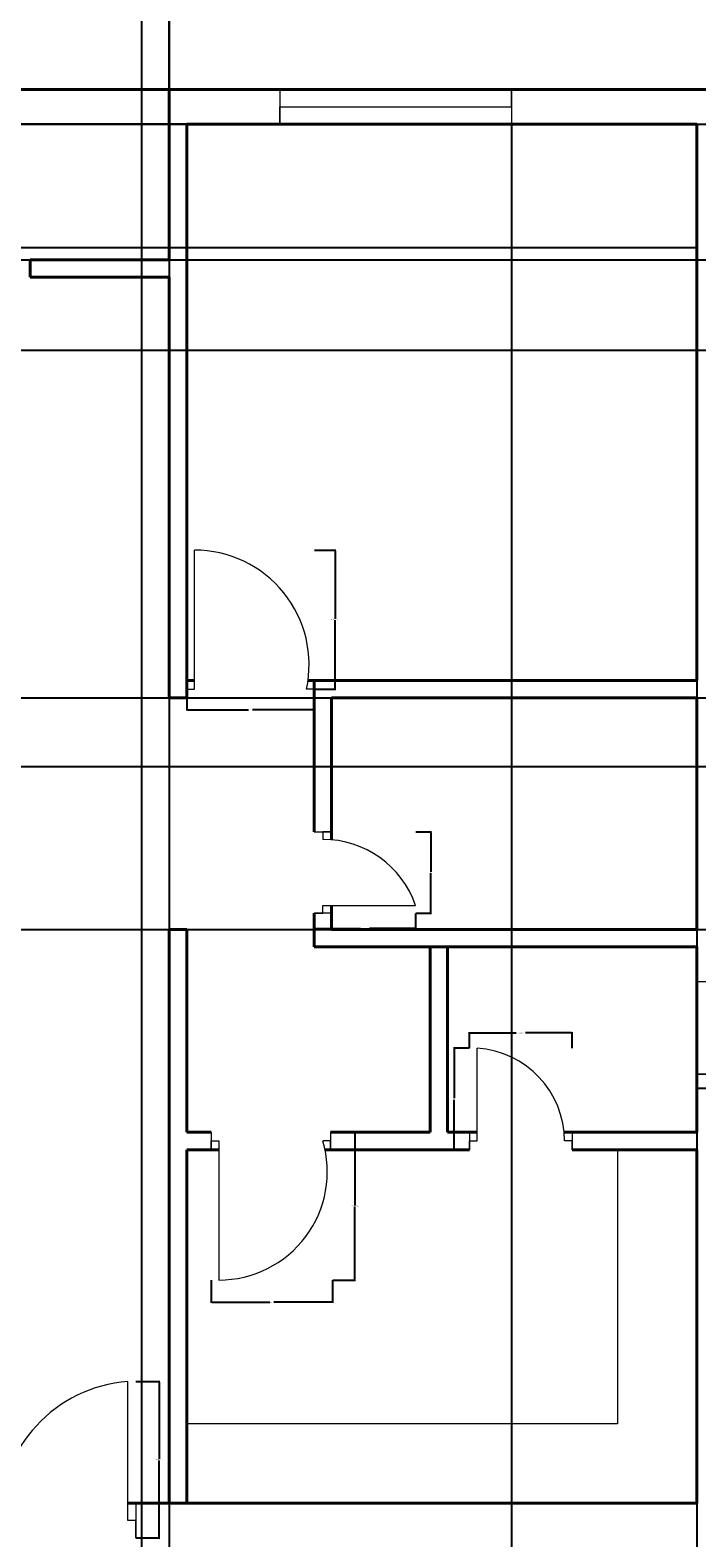
# Model space of a CAD drawing. Units: inches. Extents: x 1355 to 2746, y 1171 to 2751.
# Tile 17 of 24: x 2325 to 2497, y 1764 to 2155. Entities that reach past the tile are written whole.
import ezdxf

# ---------------------------------------------------------------- set-up
doc = ezdxf.new("R2010")
doc.units = ezdxf.units.IN
for name, color, linetype, lineweight in [('A-ANNO-DIMS', 2, 'Continuous', 18), ('A-DOOR', 3, 'Continuous', 20), ('A-FLOR-CASE', 30, 'Continuous', 20), ('A-GLAZ', 4, 'Continuous', 18), ('A-WALL', 7, 'Continuous', 40)]:
    doc.layers.add(name, color=color, linetype=linetype, lineweight=lineweight)
doc.styles.get("Standard").update_dxf_attribs({"font": 'arial.ttf'})
doc.dimstyles.get("Standard").update_dxf_attribs({"dimtxt": 0.18, "dimasz": 0.18, "dimexe": 0.18, "dimexo": 0.0625, "dimgap": 0.09, "dimtad": 0, "dimtih": 1, "dimtoh": 1, "dimdec": 4, "dimzin": 0, "dimdsep": 46, "dimtxsty": 'Standard', "dimcen": 0.09, "dimadec": 0, "dimazin": 0, "dimtfac": 1, "dimtdec": 4, "dimtofl": 0, "dimtmove": 0, "dimatfit": 3, "dimfxl": 1, "dimtolj": 1, "dimtzin": 0, "dimarcsym": 0})

# ---------------------------------------------------------------- blocks, each defined once
blk = doc.blocks.new('WINDOW-PLAN-24-2')
for p, q in [((0, 24), (9, 24)), ((9, 24), (4.5, 24)), ((4.5, 24), (4.5, 0)), ((4.5, 0), (0, 0)), ((0, 0), (0, 0)), ((0, 0), (9, 0))]:
    blk.add_line(p, q)
blk = doc.blocks.new('WINDOW-PLAN-60')
for p, q in [((0, 60), (9, 60)), ((9, 60), (4.5, 60)), ((4.5, 60), (4.5, 0)), ((4.5, 0), (0, 0)), ((0, 0), (9, 0))]:
    blk.add_line(p, q)
blk = doc.blocks.new('DOOR-ENTRY-N')
for p, q in [((35.29, 4.5), (35.29, 40.5)), ((0, 9), (0, 0)), ((37.29, 9), (37.29, 0)), ((0, 0), (0, 4.5)), ((0, 4.5), (2, 4.5)), ((37.29, 4.5), (35.29, 4.5)), ((37.29, 0), (37.29, 4.5))]:
    blk.add_line(p, q)
blk.add_arc((38.11, 4.5), 36.11, 94.4716, 180)
blk = doc.blocks.new('DOOR-UTILITY-N')
for p, q in [((2, 2.25), (2, 26.25)), ((0, 4.5), (0, 0)), ((26.56, 4.5), (26.56, 0)), ((0, 0), (0, 2.25)), ((0, 2.25), (2, 2.25)), ((26.56, 2.25), (24.56, 2.25)), ((26.56, 0), (26.56, 2.25))]:
    blk.add_line(p, q)
blk.add_arc((0.51, 2.25), 24.05, 0, 86.4557)
blk = doc.blocks.new('DOOR-KITCHEN-N')
for p, q in [((0, 38.25), (0, 33.75)), ((0, 33.75), (0, 36)), ((0, 36), (2, 36)), ((2, 36), (2, 0)), ((30.9, 36), (28.9, 36)), ((30.9, 38.25), (30.9, 33.75)), ((30.9, 33.75), (30.9, 36))]:
    blk.add_line(p, q)
blk.add_arc((2, 28.05), 28.05, 270, 16.4594)
blk = doc.blocks.new('DOOR-BED-NE')
for p, q in [((2, 0), (2, 36)), ((33, 0.01), (31, 0.01)), ((0, 0), (2, 0))]:
    blk.add_line(p, q)
blk.add_arc((2, 6.32), 29.68, 347.7257, 90)
blk = doc.blocks.new('DOOR-WC-NE')
for p, q in [((0, 21.08), (4.5, 21.08)), ((4.5, 21.08), (2.25, 21.08)), ((2.25, 21.08), (2.25, 19.08)), ((4.5, 0), (0, 0)), ((0, 0), (2.25, 0)), ((2.25, 0), (2.25, 2)), ((2.25, 2), (26.25, 2))]:
    blk.add_line(p, q)
blk.add_arc((2.25, -6.32), 25.4, 19.1149, 90)
blk = doc.blocks.new('*D50')
at = {"layer": 'A-ANNO-DIMS', "color": 0, "lineweight": -2, "transparency": 16777216}
for p, q in [((2497.39, 1884.27), (2497.39, 1880.55)), ((2506.39, 1884.27), (2506.39, 1880.55)), ((2497.57, 1880.73), (2501.43, 1880.73)), ((2506.21, 1880.73), (2502.35, 1880.73))]:
    blk.add_line(p, q, dxfattribs=at)
at = {"layer": 'A-ANNO-DIMS', "color": 0, "transparency": 16777216}
for points in [[(2497.57, 1880.76), (2497.57, 1880.7), (2497.39, 1880.73)], [(2506.21, 1880.76), (2506.21, 1880.7), (2506.39, 1880.73)]]:
    blk.add_solid(points, dxfattribs=at)
at = {"layer": 'Defpoints', "color": 0, "transparency": 16777216}
for p in [(2497.39, 1884.33), (2506.39, 1884.33), (2506.39, 1880.73)]:
    blk.add_point(p, dxfattribs=at)
at = {"layer": 'A-ANNO-DIMS', "color": 0, "transparency": 16777216, "insert": (2501.89, 1880.73), "char_height": 0.18, "attachment_point": 5}
blk.add_mtext('\\A1;9 TYP.', dxfattribs=at)
blk = doc.blocks.new('*D55')
at = {"layer": 'A-ANNO-DIMS', "color": 0, "lineweight": -2, "transparency": 16777216}
for p, q in [((2352.26, 1804.8), (2358.45, 1804.8)), ((2358.27, 1804.62), (2358.27, 1784.73)), ((2358.27, 1764.48), (2358.27, 1784.37)), ((2352.26, 1764.3), (2358.45, 1764.3))]:
    blk.add_line(p, q, dxfattribs=at)
at = {"layer": 'A-ANNO-DIMS', "color": 0, "transparency": 16777216}
for points in [[(2358.24, 1804.62), (2358.3, 1804.62), (2358.27, 1804.8)], [(2358.24, 1764.48), (2358.3, 1764.48), (2358.27, 1764.3)]]:
    blk.add_solid(points, dxfattribs=at)
at = {"layer": 'Defpoints', "color": 0, "transparency": 16777216}
for p in [(2352.2, 1804.8), (2358.27, 1804.8), (2352.2, 1764.3)]:
    blk.add_point(p, dxfattribs=at)
at = {"layer": 'A-ANNO-DIMS', "color": 0, "transparency": 16777216, "insert": (2358.27, 1784.55), "char_height": 0.18, "attachment_point": 5}
blk.add_mtext('\\A1;ENTRY DOOR 41 TYP.', dxfattribs=at)
blk = doc.blocks.new('*D57')
at = {"layer": 'A-ANNO-DIMS', "color": 0, "lineweight": -2, "transparency": 16777216}
for p, q in [((2438.58, 1891.11), (2438.58, 1895.22)), ((2438.76, 1895.04), (2450.62, 1895.04)), ((2464.96, 1895.04), (2453.1, 1895.04)), ((2465.14, 1891.11), (2465.14, 1895.22))]:
    blk.add_line(p, q, dxfattribs=at)
at = {"layer": 'A-ANNO-DIMS', "color": 0, "transparency": 16777216}
for points in [[(2438.76, 1895.07), (2438.76, 1895.01), (2438.58, 1895.04)], [(2464.96, 1895.07), (2464.96, 1895.01), (2465.14, 1895.04)]]:
    blk.add_solid(points, dxfattribs=at)
at = {"layer": 'Defpoints', "color": 0, "transparency": 16777216}
for p in [(2465.14, 1895.04), (2438.58, 1891.05), (2465.14, 1891.05)]:
    blk.add_point(p, dxfattribs=at)
at = {"layer": 'A-ANNO-DIMS', "color": 0, "transparency": 16777216, "insert": (2451.86, 1895.04), "char_height": 0.18, "attachment_point": 5}
blk.add_mtext('\\A1;UTIL DOOR 27 TYP.', dxfattribs=at)
blk = doc.blocks.new('*D58')
at = {"layer": 'A-ANNO-DIMS', "color": 0, "lineweight": -2, "transparency": 16777216}
for p, q in [((2438.52, 1891.05), (2434.42, 1891.05)), ((2434.6, 1890.87), (2434.6, 1878.11)), ((2434.6, 1864.98), (2434.6, 1877.74)), ((2438.52, 1864.8), (2434.42, 1864.8))]:
    blk.add_line(p, q, dxfattribs=at)
at = {"layer": 'A-ANNO-DIMS', "color": 0, "transparency": 16777216}
for points in [[(2434.57, 1890.87), (2434.63, 1890.87), (2434.6, 1891.05)], [(2434.57, 1864.98), (2434.63, 1864.98), (2434.6, 1864.8)]]:
    blk.add_solid(points, dxfattribs=at)
at = {"layer": 'Defpoints', "color": 0, "transparency": 16777216}
for p in [(2434.6, 1891.05), (2438.58, 1891.05), (2438.58, 1864.8)]:
    blk.add_point(p, dxfattribs=at)
at = {"layer": 'A-ANNO-DIMS', "color": 0, "transparency": 16777216, "insert": (2434.6, 1877.93), "char_height": 0.18, "attachment_point": 5}
blk.add_mtext('\\A1;26 TYP.', dxfattribs=at)
blk = doc.blocks.new('*D59')
at = {"layer": 'A-ANNO-DIMS', "color": 0, "lineweight": -2, "transparency": 16777216}
for p, q in [((2403.21, 1869.3), (2409.06, 1869.3)), ((2408.88, 1869.12), (2408.88, 1850.36)), ((2408.88, 1831.23), (2408.88, 1849.99)), ((2403.21, 1831.05), (2409.06, 1831.05))]:
    blk.add_line(p, q, dxfattribs=at)
at = {"layer": 'A-ANNO-DIMS', "color": 0, "transparency": 16777216}
for points in [[(2408.85, 1869.12), (2408.91, 1869.12), (2408.88, 1869.3)], [(2408.85, 1831.23), (2408.91, 1831.23), (2408.88, 1831.05)]]:
    blk.add_solid(points, dxfattribs=at)
at = {"layer": 'Defpoints', "color": 0, "transparency": 16777216}
for p in [(2403.14, 1869.3), (2408.88, 1869.3), (2403.14, 1831.05)]:
    blk.add_point(p, dxfattribs=at)
at = {"layer": 'A-ANNO-DIMS', "color": 0, "transparency": 16777216, "insert": (2408.88, 1850.18), "char_height": 0.18, "attachment_point": 5}
blk.add_mtext('\\A1;KIT DOOR 38 TYP.', dxfattribs=at)
blk = doc.blocks.new('*D60')
at = {"layer": 'A-ANNO-DIMS', "color": 0, "lineweight": -2, "transparency": 16777216}
for p, q in [((2371.73, 1830.99), (2371.73, 1825.13)), ((2403.14, 1830.99), (2403.14, 1825.13)), ((2371.91, 1825.31), (2386.91, 1825.31)), ((2402.96, 1825.31), (2387.97, 1825.31))]:
    blk.add_line(p, q, dxfattribs=at)
at = {"layer": 'A-ANNO-DIMS', "color": 0, "transparency": 16777216}
for points in [[(2371.91, 1825.34), (2371.91, 1825.28), (2371.73, 1825.31)], [(2402.96, 1825.34), (2402.96, 1825.28), (2403.14, 1825.31)]]:
    blk.add_solid(points, dxfattribs=at)
at = {"layer": 'Defpoints', "color": 0, "transparency": 16777216}
for p in [(2371.73, 1831.05), (2403.14, 1831.05), (2403.14, 1825.31)]:
    blk.add_point(p, dxfattribs=at)
at = {"layer": 'A-ANNO-DIMS', "color": 0, "transparency": 16777216, "insert": (2387.44, 1825.31), "char_height": 0.18, "attachment_point": 5}
blk.add_mtext('\\A1;31 TYP.', dxfattribs=at)
blk = doc.blocks.new('*D77')
at = {"layer": 'A-ANNO-DIMS', "color": 0, "lineweight": -2, "transparency": 16777216}
for p, q in [((2398.45, 2020.05), (2403.97, 2020.05)), ((2403.79, 2019.87), (2403.79, 2002.24)), ((2403.79, 1984.23), (2403.79, 2001.87)), ((2398.45, 1984.05), (2403.97, 1984.05))]:
    blk.add_line(p, q, dxfattribs=at)
at = {"layer": 'A-ANNO-DIMS', "color": 0, "transparency": 16777216}
for points in [[(2403.76, 2019.87), (2403.82, 2019.87), (2403.79, 2020.05)], [(2403.76, 1984.23), (2403.82, 1984.23), (2403.79, 1984.05)]]:
    blk.add_solid(points, dxfattribs=at)
at = {"layer": 'Defpoints', "color": 0, "transparency": 16777216}
for p in [(2398.39, 2020.05), (2403.79, 2020.05), (2398.39, 1984.05)]:
    blk.add_point(p, dxfattribs=at)
at = {"layer": 'A-ANNO-DIMS', "color": 0, "transparency": 16777216, "insert": (2403.79, 2002.05), "char_height": 0.18, "attachment_point": 5}
blk.add_mtext('\\A1;BED DOOR 36 TYP.', dxfattribs=at)
blk = doc.blocks.new('*D78')
at = {"layer": 'A-ANNO-DIMS', "color": 0, "lineweight": -2, "transparency": 16777216}
for p, q in [((2365.39, 1983.99), (2365.39, 1978.47)), ((2398.39, 1983.99), (2398.39, 1978.47)), ((2365.57, 1978.65), (2381.36, 1978.65)), ((2398.21, 1978.65), (2382.42, 1978.65))]:
    blk.add_line(p, q, dxfattribs=at)
at = {"layer": 'A-ANNO-DIMS', "color": 0, "transparency": 16777216}
for points in [[(2365.57, 1978.68), (2365.57, 1978.62), (2365.39, 1978.65)], [(2398.21, 1978.68), (2398.21, 1978.62), (2398.39, 1978.65)]]:
    blk.add_solid(points, dxfattribs=at)
at = {"layer": 'Defpoints', "color": 0, "transparency": 16777216}
for p in [(2365.39, 1984.05), (2398.39, 1984.05), (2398.39, 1978.65)]:
    blk.add_point(p, dxfattribs=at)
at = {"layer": 'A-ANNO-DIMS', "color": 0, "transparency": 16777216, "insert": (2381.89, 1978.65), "char_height": 0.18, "attachment_point": 5}
blk.add_mtext('\\A1;33 TYP.', dxfattribs=at)
blk = doc.blocks.new('*D79')
at = {"layer": 'A-ANNO-DIMS', "color": 0, "lineweight": -2, "transparency": 16777216}
for p, q in [((2398.39, 1925.99), (2398.39, 1921.93)), ((2424.64, 1925.99), (2424.64, 1921.93)), ((2398.57, 1922.11), (2410.33, 1922.11)), ((2424.46, 1922.11), (2412.7, 1922.11))]:
    blk.add_line(p, q, dxfattribs=at)
at = {"layer": 'A-ANNO-DIMS', "color": 0, "transparency": 16777216}
for points in [[(2398.57, 1922.14), (2398.57, 1922.08), (2398.39, 1922.11)], [(2424.46, 1922.14), (2424.46, 1922.08), (2424.64, 1922.11)]]:
    blk.add_solid(points, dxfattribs=at)
at = {"layer": 'Defpoints', "color": 0, "transparency": 16777216}
for p in [(2398.39, 1926.05), (2424.64, 1926.05), (2424.64, 1922.11)]:
    blk.add_point(p, dxfattribs=at)
at = {"layer": 'A-ANNO-DIMS', "color": 0, "transparency": 16777216, "insert": (2411.52, 1922.11), "char_height": 0.18, "attachment_point": 5}
blk.add_mtext('\\A1;WC DOOR 26 TYP.', dxfattribs=at)
blk = doc.blocks.new('*D80')
at = {"layer": 'A-ANNO-DIMS', "color": 0, "lineweight": -2, "transparency": 16777216}
for p, q in [((2424.7, 1947.13), (2428.76, 1947.13)), ((2428.58, 1946.95), (2428.58, 1936.77)), ((2428.58, 1926.23), (2428.58, 1936.41)), ((2424.7, 1926.05), (2428.76, 1926.05))]:
    blk.add_line(p, q, dxfattribs=at)
at = {"layer": 'A-ANNO-DIMS', "color": 0, "transparency": 16777216}
for points in [[(2428.55, 1946.95), (2428.61, 1946.95), (2428.58, 1947.13)], [(2428.55, 1926.23), (2428.61, 1926.23), (2428.58, 1926.05)]]:
    blk.add_solid(points, dxfattribs=at)
at = {"layer": 'Defpoints', "color": 0, "transparency": 16777216}
for p in [(2424.64, 1947.13), (2428.58, 1947.13), (2424.64, 1926.05)]:
    blk.add_point(p, dxfattribs=at)
at = {"layer": 'A-ANNO-DIMS', "color": 0, "transparency": 16777216, "insert": (2428.58, 1936.59), "char_height": 0.18, "attachment_point": 5}
blk.add_mtext('\\A1;21 TYP.', dxfattribs=at)
blk = doc.blocks.new('*D100')
at = {"layer": 'A-ANNO-DIMS', "color": 0, "lineweight": -2, "transparency": 16777216}
for p, q in [((2225.89, 2139.36), (2225.89, 2716.58)), ((2226.07, 2716.4), (2293.11, 2716.4)), ((2360.71, 2716.4), (2293.67, 2716.4)), ((2360.89, 2139.36), (2360.89, 2716.58))]:
    blk.add_line(p, q, dxfattribs=at)
at = {"layer": 'A-ANNO-DIMS', "color": 0, "transparency": 16777216}
for points in [[(2226.07, 2716.43), (2226.07, 2716.37), (2225.89, 2716.4)], [(2360.71, 2716.43), (2360.71, 2716.37), (2360.89, 2716.4)]]:
    blk.add_solid(points, dxfattribs=at)
at = {"layer": 'Defpoints', "color": 0, "transparency": 16777216}
for p in [(2360.89, 2716.4), (2225.89, 2139.3), (2360.89, 2139.3)]:
    blk.add_point(p, dxfattribs=at)
at = {"layer": 'A-ANNO-DIMS', "color": 0, "transparency": 16777216, "insert": (2293.39, 2716.4), "char_height": 0.18, "attachment_point": 5}
blk.add_mtext('\\A1;135', dxfattribs=at)
blk = doc.blocks.new('*D101')
at = {"layer": 'A-ANNO-DIMS', "color": 0, "lineweight": -2, "transparency": 16777216}
for p, q in [((2360.89, 2139.36), (2360.89, 2716.58)), ((2361.07, 2716.4), (2433.25, 2716.4)), ((2506.21, 2716.4), (2434.03, 2716.4)), ((2506.39, 2139.36), (2506.39, 2716.58))]:
    blk.add_line(p, q, dxfattribs=at)
at = {"layer": 'A-ANNO-DIMS', "color": 0, "transparency": 16777216}
for points in [[(2361.07, 2716.43), (2361.07, 2716.37), (2360.89, 2716.4)], [(2506.21, 2716.43), (2506.21, 2716.37), (2506.39, 2716.4)]]:
    blk.add_solid(points, dxfattribs=at)
at = {"layer": 'Defpoints', "color": 0, "transparency": 16777216}
for p in [(2506.39, 2716.4), (2360.89, 2139.3), (2506.39, 2139.3)]:
    blk.add_point(p, dxfattribs=at)
at = {"layer": 'A-ANNO-DIMS', "color": 0, "transparency": 16777216, "insert": (2433.64, 2716.4), "char_height": 0.18, "attachment_point": 5}
blk.add_mtext('\\A1;145.5', dxfattribs=at)
blk = doc.blocks.new('*D109')
at = {"layer": 'A-ANNO-DIMS', "color": 0, "lineweight": -2, "transparency": 16777216}
for p, q in [((2449.47, 2130.24), (2449.47, 1171.06)), ((2497.39, 2130.24), (2497.39, 1171.06)), ((2449.65, 1171.24), (2473.04, 1171.24)), ((2497.21, 1171.24), (2473.83, 1171.24))]:
    blk.add_line(p, q, dxfattribs=at)
at = {"layer": 'A-ANNO-DIMS', "color": 0, "transparency": 16777216}
for points in [[(2449.65, 1171.27), (2449.65, 1171.21), (2449.47, 1171.24)], [(2497.21, 1171.27), (2497.21, 1171.21), (2497.39, 1171.24)]]:
    blk.add_solid(points, dxfattribs=at)
at = {"layer": 'Defpoints', "color": 0, "transparency": 16777216}
for p in [(2449.47, 2130.3), (2497.39, 2130.3), (2497.39, 1171.24)]:
    blk.add_point(p, dxfattribs=at)
at = {"layer": 'A-ANNO-DIMS', "color": 0, "transparency": 16777216, "insert": (2473.43, 1171.24), "char_height": 0.18, "attachment_point": 5}
blk.add_mtext('\\A1;47.92', dxfattribs=at)
blk = doc.blocks.new('*D110')
at = {"layer": 'A-ANNO-DIMS', "color": 0, "lineweight": -2, "transparency": 16777216}
for p, q in [((2089.45, 2130.3), (2648.07, 2130.3)), ((2647.89, 2130.12), (2647.89, 2101.25)), ((2647.89, 2072.02), (2647.89, 2100.89)), ((2089.45, 2071.84), (2648.07, 2071.84))]:
    blk.add_line(p, q, dxfattribs=at)
at = {"layer": 'A-ANNO-DIMS', "color": 0, "transparency": 16777216}
for points in [[(2647.86, 2130.12), (2647.92, 2130.12), (2647.89, 2130.3)], [(2647.86, 2072.02), (2647.92, 2072.02), (2647.89, 2071.84)]]:
    blk.add_solid(points, dxfattribs=at)
at = {"layer": 'Defpoints', "color": 0, "transparency": 16777216}
for p in [(2089.39, 2130.3), (2647.89, 2130.3), (2089.39, 2071.84)]:
    blk.add_point(p, dxfattribs=at)
at = {"layer": 'A-ANNO-DIMS', "color": 0, "transparency": 16777216, "insert": (2647.89, 2101.07), "char_height": 0.18, "attachment_point": 5}
blk.add_mtext('\\A1;58.46', dxfattribs=at)
blk = doc.blocks.new('*D111')
at = {"layer": 'A-ANNO-DIMS', "color": 0, "lineweight": -2, "transparency": 16777216}
for p, q in [((2497.33, 2130.3), (1407.53, 2130.3)), ((1407.71, 2130.12), (1407.71, 2114.5)), ((1407.71, 2098.51), (1407.71, 2114.14)), ((2497.33, 2098.33), (1407.53, 2098.33))]:
    blk.add_line(p, q, dxfattribs=at)
at = {"layer": 'A-ANNO-DIMS', "color": 0, "transparency": 16777216}
for points in [[(1407.68, 2130.12), (1407.74, 2130.12), (1407.71, 2130.3)], [(1407.68, 2098.51), (1407.74, 2098.51), (1407.71, 2098.33)]]:
    blk.add_solid(points, dxfattribs=at)
at = {"layer": 'Defpoints', "color": 0, "transparency": 16777216}
for p in [(1407.71, 2130.3), (2497.39, 2130.3), (2497.39, 2098.33)]:
    blk.add_point(p, dxfattribs=at)
at = {"layer": 'A-ANNO-DIMS', "color": 0, "transparency": 16777216, "insert": (1407.71, 2114.32), "char_height": 0.18, "attachment_point": 5}
blk.add_mtext('\\A1;31.97', dxfattribs=at)
blk = doc.blocks.new('*D113')
at = {"layer": 'A-ANNO-DIMS', "color": 0, "lineweight": -2, "transparency": 16777216}
for p, q in [((2225.95, 2139.3), (2648.07, 2139.3)), ((2647.89, 2139.12), (2647.89, 2117.44)), ((2647.89, 2095.4), (2647.89, 2117.08)), ((2225.95, 2095.22), (2648.07, 2095.22))]:
    blk.add_line(p, q, dxfattribs=at)
at = {"layer": 'A-ANNO-DIMS', "color": 0, "transparency": 16777216}
for points in [[(2647.86, 2139.12), (2647.92, 2139.12), (2647.89, 2139.3)], [(2647.86, 2095.4), (2647.92, 2095.4), (2647.89, 2095.22)]]:
    blk.add_solid(points, dxfattribs=at)
at = {"layer": 'Defpoints', "color": 0, "transparency": 16777216}
for p in [(2225.89, 2139.3), (2647.89, 2139.3), (2225.89, 2095.22)]:
    blk.add_point(p, dxfattribs=at)
at = {"layer": 'A-ANNO-DIMS', "color": 0, "transparency": 16777216, "insert": (2647.89, 2117.26), "char_height": 0.18, "attachment_point": 5}
blk.add_mtext('\\A1;44.08', dxfattribs=at)
blk = doc.blocks.new('*D126')
at = {"layer": 'A-ANNO-DIMS', "color": 0, "lineweight": -2, "transparency": 16777216}
for p, q in [((2080.39, 2219.34), (2080.39, 1171.06)), ((2506.39, 2219.34), (2506.39, 1171.06)), ((2080.57, 1171.24), (2293.1, 1171.24)), ((2506.21, 1171.24), (2293.68, 1171.24))]:
    blk.add_line(p, q, dxfattribs=at)
at = {"layer": 'A-ANNO-DIMS', "color": 0, "transparency": 16777216}
for points in [[(2080.57, 1171.27), (2080.57, 1171.21), (2080.39, 1171.24)], [(2506.21, 1171.27), (2506.21, 1171.21), (2506.39, 1171.24)]]:
    blk.add_solid(points, dxfattribs=at)
at = {"layer": 'Defpoints', "color": 0, "transparency": 16777216}
for p in [(2080.39, 2219.4), (2506.39, 2219.4), (2506.39, 1171.24)]:
    blk.add_point(p, dxfattribs=at)
at = {"layer": 'A-ANNO-DIMS', "color": 0, "transparency": 16777216, "insert": (2293.39, 1171.24), "char_height": 0.18, "attachment_point": 5}
blk.add_mtext('\\A1;426', dxfattribs=at)
blk = doc.blocks.new('*D134')
at = {"layer": 'A-ANNO-DIMS', "color": 0, "lineweight": -2, "transparency": 16777216}
for p, q in [((2353.71, 2477.34), (2353.71, 1171.06)), ((2360.89, 2477.34), (2360.89, 1171.06)), ((2353.89, 1171.24), (2356.92, 1171.24)), ((2360.71, 1171.24), (2357.68, 1171.24))]:
    blk.add_line(p, q, dxfattribs=at)
at = {"layer": 'A-ANNO-DIMS', "color": 0, "transparency": 16777216}
for points in [[(2353.89, 1171.27), (2353.89, 1171.21), (2353.71, 1171.24)], [(2360.71, 1171.27), (2360.71, 1171.21), (2360.89, 1171.24)]]:
    blk.add_solid(points, dxfattribs=at)
at = {"layer": 'Defpoints', "color": 0, "transparency": 16777216}
for p in [(2353.71, 2477.4), (2360.89, 2477.4), (2360.89, 1171.24)]:
    blk.add_point(p, dxfattribs=at)
at = {"layer": 'A-ANNO-DIMS', "color": 0, "transparency": 16777216, "insert": (2357.3, 1171.24), "char_height": 0.18, "attachment_point": 5}
blk.add_mtext('\\A1;7.181', dxfattribs=at)
blk = doc.blocks.new('*D136')
at = {"layer": 'A-ANNO-DIMS', "color": 0, "lineweight": -2, "transparency": 16777216}
for p, q in [((1618.27, 1981.8), (2648.07, 1981.8)), ((2647.89, 1981.62), (2647.89, 1951.98)), ((2647.89, 1921.98), (2647.89, 1951.62)), ((1618.27, 1921.8), (2648.07, 1921.8))]:
    blk.add_line(p, q, dxfattribs=at)
at = {"layer": 'A-ANNO-DIMS', "color": 0, "transparency": 16777216}
for points in [[(2647.86, 1981.62), (2647.92, 1981.62), (2647.89, 1981.8)], [(2647.86, 1921.98), (2647.92, 1921.98), (2647.89, 1921.8)]]:
    blk.add_solid(points, dxfattribs=at)
at = {"layer": 'Defpoints', "color": 0, "transparency": 16777216}
for p in [(1618.21, 1981.8), (2647.89, 1981.8), (1618.21, 1921.8)]:
    blk.add_point(p, dxfattribs=at)
at = {"layer": 'A-ANNO-DIMS', "color": 0, "transparency": 16777216, "insert": (2647.89, 1951.8), "char_height": 0.18, "attachment_point": 5}
blk.add_mtext('\\A1;60', dxfattribs=at)
blk = doc.blocks.new('*D139')
at = {"layer": 'A-ANNO-DIMS', "color": 0, "lineweight": -2, "transparency": 16777216}
for p, q in [((1523.77, 1981.8), (2648.07, 1981.8)), ((2647.89, 1981.62), (2647.89, 1973.09)), ((2647.89, 1964.19), (2647.89, 1972.72)), ((1548.66, 1964.01), (2648.07, 1964.01))]:
    blk.add_line(p, q, dxfattribs=at)
at = {"layer": 'A-ANNO-DIMS', "color": 0, "transparency": 16777216}
for points in [[(2647.86, 1981.62), (2647.92, 1981.62), (2647.89, 1981.8)], [(2647.86, 1964.19), (2647.92, 1964.19), (2647.89, 1964.01)]]:
    blk.add_solid(points, dxfattribs=at)
at = {"layer": 'Defpoints', "color": 0, "transparency": 16777216}
for p in [(1523.71, 1981.8), (1548.6, 1964.01), (2647.89, 1964.01)]:
    blk.add_point(p, dxfattribs=at)
at = {"layer": 'A-ANNO-DIMS', "color": 0, "transparency": 16777216, "insert": (2647.89, 1972.9), "char_height": 0.18, "attachment_point": 5}
blk.add_mtext('\\A1;17.795', dxfattribs=at)

msp = doc.modelspace()

# ---------------------------------------------------------------- linework, layer by layer
at = {"layer": 'A-FLOR-CASE'}
for p, q in [((2476.8717, 1864.8018), (2476.8717, 1793.8497)), ((2476.8717, 1793.8497), (2365.3909, 1793.8497))]:
    msp.add_line(p, q, dxfattribs=at)
at = {"layer": 'A-WALL'}
for p, q in [((2225.8909, 2139.3018), (2360.8909, 2139.3018)), ((2360.8909, 2139.3018), (2506.3909, 2139.3018)), ((2360.8909, 2130.3018), (2360.8909, 2139.3018)), ((2360.8909, 2130.3018), (2360.8909, 2095.2225)), ((2365.3909, 2130.3018), (2497.3909, 2130.3018)), ((2365.3909, 2130.3018), (2365.3909, 1986.3018)), ((2497.3909, 2130.3018), (2497.3909, 1986.3018)), ((2324.8959, 2095.2225), (2360.8909, 2095.2225)), ((2324.8959, 2095.2225), (2324.8959, 2090.7225)), ((2360.8909, 2090.7225), (2324.8959, 2090.7225)), ((2360.8909, 2090.7225), (2360.8909, 1981.8018)), ((2365.3909, 1986.3018), (2367.3909, 1986.3018)), ((2365.3909, 1986.3018), (2365.3909, 1981.8018)), ((2396.7887, 1986.3018), (2497.3909, 1986.3018)), ((2398.3909, 1947.1338), (2398.3909, 1986.3018)), ((2398.3909, 1986.3018), (2402.8909, 1986.3018)), ((2360.8909, 1981.8018), (2365.3909, 1981.8018)), ((2402.8909, 1981.8018), (2497.3909, 1981.8018)), ((2402.8909, 1981.8018), (2402.8909, 1945.034)), ((2497.3909, 1981.8018), (2497.3909, 1921.8018)), ((2398.3909, 1917.3018), (2398.3909, 1926.0511)), ((2402.8909, 1928.0511), (2402.8909, 1921.8018)), ((2360.8909, 1921.8018), (2365.3909, 1921.8018)), ((2360.8909, 1921.8018), (2360.8909, 1773.3018)), ((2365.3909, 1917.3018), (2365.3909, 1921.8018)), ((2402.8909, 1921.8018), (2497.3909, 1921.8018)), ((2365.3909, 1917.3018), (2365.3909, 1869.3018)), ((2398.3909, 1917.3018), (2497.3909, 1917.3018)), ((2432.8909, 1917.3018), (2428.3909, 1917.3018)), ((2428.3909, 1917.3018), (2428.3909, 1869.3018)), ((2432.8909, 1869.3018), (2432.8909, 1917.3018)), ((2497.3909, 1917.3018), (2497.3909, 1869.3018)), ((2497.3909, 1917.3018), (2497.3909, 1869.3018)), ((2371.7348, 1869.3018), (2365.3909, 1869.3018)), ((2428.3909, 1869.3018), (2402.6372, 1869.3018)), ((2440.5814, 1869.3018), (2432.8909, 1869.3018)), ((2497.3909, 1869.3018), (2463.0354, 1869.3018)), ((2365.3909, 1864.8018), (2365.3909, 1773.3018)), ((2365.3909, 1864.8018), (2373.7348, 1864.8018)), ((2401.2019, 1864.8018), (2428.3909, 1864.8018)), ((2428.3909, 1864.8018), (2438.5814, 1864.8018)), ((2465.1409, 1864.8018), (2497.3909, 1864.8018)), ((2497.3909, 1864.8018), (2497.3909, 1773.3018)), ((2350.1969, 1773.3018), (2497.3909, 1773.3018))]:
    msp.add_line(p, q, dxfattribs=at)

# ---------------------------------------------------------------- block references
at = {"layer": 'A-DOOR'}
for name, p in [('DOOR-BED-NE', (2365.3906, 1984.052)), ('DOOR-WC-NE', (2398.3906, 1926.051)), ('DOOR-UTILITY-N', (2438.5816, 1864.802)), ('DOOR-KITCHEN-N', (2371.7346, 1831.052)), ('DOOR-ENTRY-N', (2314.9026, 1764.302))]:
    msp.add_blockref(name, p, dxfattribs=at)
at = {"layer": 'A-GLAZ', "extrusion": (0, 0, -1), "zscale": -1, "rotation": 270}
msp.add_blockref('WINDOW-PLAN-60', (-2449.475, 2139.302), dxfattribs=at)
at = {"layer": 'A-GLAZ'}
msp.add_blockref('WINDOW-PLAN-24-2', (2497.3906, 1884.332), dxfattribs=at)

# ---------------------------------------------------------------- dimensions: what is measured, and where the dimension line sits
at = {"layer": 'A-ANNO-DIMS'}
for base, p1, p2, override, picture, middle in [((2360.8909, 2716.3999), (2225.8909, 2139.3018), (2360.8909, 2139.3018), {"dimdec": 0, "dimlfac": 1, "dimrnd": 0, "dimzin": 0, "dimdsep": 46, "dimlunit": 2}, '*D100', (2293.3909, 2716.3999)), ((2506.3909, 2716.3999), (2360.8909, 2139.3018), (2506.3909, 2139.3018), {"dimdec": 1, "dimlfac": 1, "dimrnd": 0, "dimzin": 0, "dimdsep": 46, "dimlunit": 2}, '*D101', (2433.6409, 2716.3999)), ((2360.8909, 1171.2388), (2353.71, 2477.3999), (2360.8909, 2477.3999), {"dimdec": 3, "dimlfac": 1, "dimrnd": 0, "dimzin": 0, "dimdsep": 46, "dimlunit": 2}, '*D134', (2357.3004, 1171.2388)), ((2506.3909, 1171.2388), (2080.3909, 2219.3999), (2506.3909, 2219.3999), {"dimdec": 0, "dimlfac": 1, "dimrnd": 0, "dimzin": 0, "dimdsep": 46, "dimlunit": 2}, '*D126', (2293.3909, 1171.2388)), ((2497.3909, 1171.2388), (2449.4747, 2130.3017), (2497.3909, 2130.3018), {"dimdec": 2, "dimlfac": 1, "dimrnd": 0, "dimzin": 0, "dimdsep": 46, "dimlunit": 2}, '*D109', (2473.4328, 1171.2388))]:
    dim = msp.add_linear_dim(base=base, p1=p1, p2=p2, dimstyle='Standard', override=override, dxfattribs=at)
    dim.commit()
    dim.dimension.update_dxf_attribs({"geometry": picture, "text_midpoint": middle})
for base, p1, p2, override, picture, middle in [((2647.886, 2139.3018), (2225.8909, 2095.2225), (2225.8909, 2139.3018), {"dimdec": 2, "dimlfac": 1, "dimrnd": 0, "dimzin": 0, "dimdsep": 46, "dimlunit": 2}, '*D113', (2647.886, 2117.2622)), ((1407.7083, 2130.3018), (2497.3909, 2098.3333), (2497.3909, 2130.3018), {"dimdec": 2, "dimlfac": 1, "dimrnd": 0, "dimzin": 0, "dimdsep": 46, "dimlunit": 2}, '*D111', (1407.7083, 2114.3176)), ((2647.886, 2130.3018), (2089.3909, 2071.8385), (2089.3909, 2130.3018), {"dimdec": 2, "dimlfac": 1, "dimrnd": 0, "dimzin": 0, "dimdsep": 46, "dimlunit": 2}, '*D110', (2647.886, 2101.0702)), ((2647.886, 1964.0069), (1523.7083, 1981.8018), (1548.5973, 1964.0069), {"dimdec": 3, "dimlfac": 1, "dimrnd": 0, "dimzin": 0, "dimdsep": 46, "dimlunit": 2}, '*D139', (2647.886, 1972.9044)), ((2647.886, 1981.8018), (1618.2083, 1921.8018), (1618.2083, 1981.8018), {"dimdec": 0, "dimlfac": 1, "dimrnd": 0, "dimzin": 0, "dimdsep": 46, "dimlunit": 2}, '*D136', (2647.886, 1951.8018))]:
    dim = msp.add_linear_dim(base=base, p1=p1, p2=p2, angle=90, dimstyle='Standard', override=override, dxfattribs=at)
    dim.commit()
    dim.dimension.update_dxf_attribs({"geometry": picture, "text_midpoint": middle})
for base, p1, p2, text, picture, middle in [((2403.7909, 2020.0518), (2398.3909, 1984.0518), (2398.3909, 2020.0518), 'BED DOOR <> TYP.', '*D77', (2403.7909, 2002.0518)), ((2428.5784, 1947.1338), (2424.6409, 1926.0511), (2424.6409, 1947.1338), '<> TYP.', '*D80', (2428.5784, 1936.5924)), ((2434.5975, 1891.0518), (2438.5814, 1864.8018), (2438.5814, 1891.0518), '<> TYP.', '*D58', (2434.5975, 1877.9268)), ((2408.8812, 1869.3018), (2403.1437, 1831.0518), (2403.1437, 1869.3018), 'KIT DOOR <> TYP.', '*D59', (2408.8812, 1850.1768)), ((2358.2719197084, 1804.8018275923), (2352.1969197084, 1764.3018275923), (2352.1969197084, 1804.8018275923), 'ENTRY DOOR <> TYP.', '*D55', (2358.2719197084, 1784.5518275923))]:
    dim = msp.add_linear_dim(base=base, p1=p1, p2=p2, angle=90, text=text, dimstyle='Standard', override={"dimdec": 0, "dimlfac": 1, "dimrnd": 0, "dimzin": 0, "dimdsep": 46, "dimlunit": 2}, dxfattribs=at)
    dim.commit()
    dim.dimension.update_dxf_attribs({"geometry": picture, "text_midpoint": middle})
for base, p1, p2, text, picture, middle in [((2398.3909, 1978.6518), (2365.3909, 1984.0518), (2398.3909, 1984.0518), '<> TYP.', '*D78', (2381.8909, 1978.6518)), ((2424.6409, 1922.1136), (2398.3909, 1926.0511), (2424.6409, 1926.0511), 'WC DOOR <> TYP.', '*D79', (2411.5159, 1922.1136)), ((2465.1409, 1895.0357), (2438.5814, 1891.0518), (2465.1409, 1891.0518), 'UTIL DOOR <> TYP.', '*D57', (2451.8612, 1895.0357)), ((2506.3909, 1880.7321), (2497.3909, 1884.3321), (2506.3909, 1884.3321), '<> TYP.', '*D50', (2501.8909, 1880.7321)), ((2403.1437, 1825.3143), (2371.7348, 1831.0518), (2403.1437, 1831.0518), '<> TYP.', '*D60', (2387.4393, 1825.3143))]:
    dim = msp.add_linear_dim(base=base, p1=p1, p2=p2, text=text, dimstyle='Standard', override={"dimdec": 0, "dimlfac": 1, "dimrnd": 0, "dimzin": 0, "dimdsep": 46, "dimlunit": 2}, dxfattribs=at)
    dim.commit()
    dim.dimension.update_dxf_attribs({"geometry": picture, "text_midpoint": middle})

doc.saveas('drawing.dxf')
